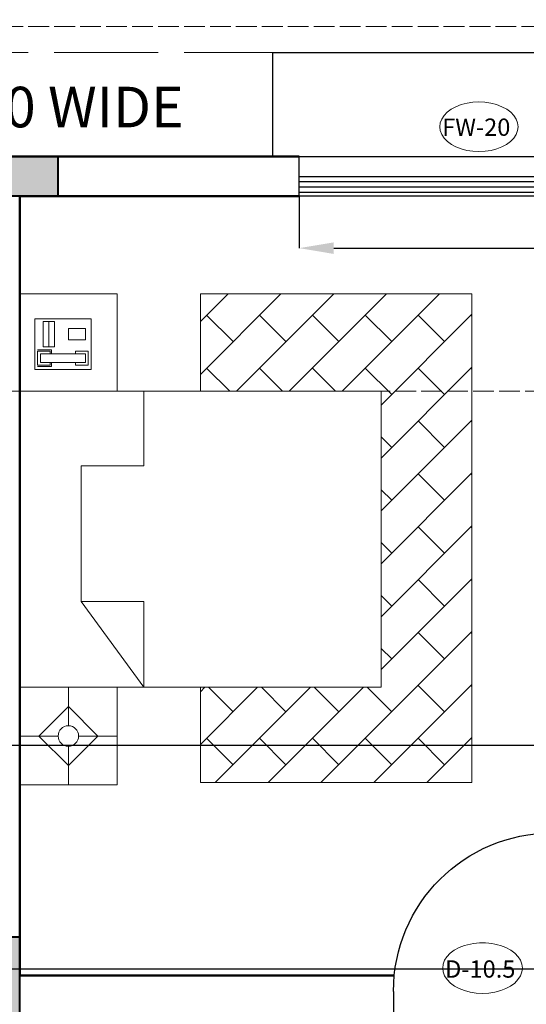
# Model space of a CAD drawing. Units: inches. Extents: x 22626 to 57351, y 2118 to 36234.
# Tile 8 of 10: x 41227 to 44155, y 23360 to 29046. Entities that reach past the tile are written whole.
import ezdxf

# ---------------------------------------------------------------- set-up
doc = ezdxf.new("R2010")
doc.units = ezdxf.units.IN
doc.header["$MEASUREMENT"] = 0
doc.linetypes.add('ACAD_ISO02W100', pattern=[15, 12, -3])
for name, color, linetype, lineweight in [('A-ANNO-DIMS', 130, 'Continuous', 18), ('A-ANNO-IDEN', 130, 'Continuous', 15), ('A-AREA-IDEN', 130, 'Continuous', 18), ('A-COLS', 7, 'Continuous', 40), ('A-ROOF', 80, 'Continuous', 25), ('A-ROOF-OVHD', 80, 'ACAD_ISO02W100', 18), ('A-WALL', 80, 'Continuous', 50), ('DOORS', 32, 'Continuous', 25), ('FURNITURE', 30, 'Continuous', 18), ('WINDOWS', 212, 'Continuous', 25)]:
    doc.layers.add(name, color=color, linetype=linetype, lineweight=lineweight)
doc.layers.add('A-SECT', color=2, linetype='ACAD_ISO02W100', lineweight=18, true_color=0xf1eb1f)
doc.styles.get("Standard").update_dxf_attribs({"font": 'arial.ttf'})
doc.dimstyles.get("Standard").update_dxf_attribs({"dimtxt": 150, "dimasz": 200, "dimexe": 0.18, "dimexo": 0.0625, "dimgap": 0.09, "dimtad": 0, "dimtih": 1, "dimtoh": 1, "dimdec": 0, "dimzin": 0, "dimdsep": 46, "dimtxsty": 'Standard', "dimcen": 0.09, "dimadec": 0, "dimazin": 0, "dimtfac": 1, "dimtdec": 0, "dimtofl": 0, "dimtmove": 0, "dimatfit": 3, "dimfxl": 1, "dimtolj": 1, "dimtzin": 0, "dimarcsym": 0})

# ---------------------------------------------------------------- blocks, each defined once
blk = doc.blocks.new('*U7')
for p, q in [((0, 0), (-1e-16, -5.999999999999999)), ((40, -6e-16), (40, -6))]:
    blk.add_line(p, q)
blk.add_lwpolyline([(0, 0), (5.6e-15, 40), (1.750000000000007, 40), (1.749999999999998, -7e-16)], close=True)
blk.add_arc((0, 0), 40, 0, 90)
blk = doc.blocks.new('Phone - Desk')
for p, q in [((-4.5, -5), (-4.5, 5)), ((-4.5, 5), (4.5, 5)), ((-4, 4.5), (-4, 2)), ((-3.75, 4.5), (-3.75, 2.25)), ((-1.25, 4.5), (-3.75, 4.5)), ((-3.25, 4), (-3.25, -4)), ((-3.25, 4), (-1.75, 4)), ((-1.75, -4), (-1.75, 4)), ((-1.25, 2.25), (-1.25, 4.5)), ((-1, 2), (-1, 4.5)), ((4, 3.5), (-0.5, 3.5)), ((-0.5, 3.5), (-0.5, 1.5)), ((4, 1.5), (4, 3.5)), ((4.5, 5), (4.5, -5)), ((-4, 2), (-3.25, 2)), ((-3.75, 2.25), (-3.25, 2.25)), ((-1.75, 2.25), (-1.25, 2.25)), ((-1.75, 2), (-1, 2)), ((-0.5, 2.5), (4, 2.5)), ((-0.5, 1.5), (4, 1.5)), ((2.75, -1), (0.75, -1)), ((0.75, -1), (0.75, -4)), ((2.75, -4), (2.75, -1)), ((-3.75, -2.25), (-3.25, -2.25)), ((-3.75, -4.5), (-3.75, -2.25)), ((-1.75, -2.25), (-1.25, -2.25)), ((-1.25, -2.25), (-1.25, -4.5)), ((4.5, -5), (-4.5, -5)), ((-1.25, -4.5), (-3.75, -4.5)), ((-3.25, -4), (-1.75, -4)), ((0.75, -4), (2.75, -4))]:
    blk.add_line(p, q)
blk = doc.blocks.new('BED')
h = blk.add_hatch()
h.set_pattern_fill('AR-B816', color=256, scale=27, angle=45)
h.set_pattern_definition([(45, (0, 0), (-152.7350647362943, 152.7350647362943), []), (135, (0, 0), (-305.4701294725885, 2.84e-14), [216, -216])])
h.paths.add_polyline_path([(36405.44497120028, 26900.74076162673), (36405.44497120028, 25190.72745343954), (35361.43700757947, 25190.72745343954), (35361.43700757947, 24640.23607026327), (36930.74850823512, 24640.23607026327), (36930.74850823512, 25190.72745343954), (36930.74850823512, 27463.39567013072), (36405.44497120028, 27463.39567013072), (35361.43700757947, 27463.39567013072), (35361.43700757947, 26900.74076162673)])
for p, q in [((35361.43700757947, 26900.74076162673), (35361.43700757947, 27463.39567013072)), ((35361.43700757947, 27463.39567013072), (36405.44497120028, 27463.39567013072)), ((36405.44497120028, 27463.39567013072), (36930.74850823512, 27463.39567013072)), ((36930.74850823512, 27463.39567013072), (36930.74850823512, 25190.72745343954)), ((35034.9123526114, 26900.74076162673), (35034.9123526114, 26469.4222770051)), ((34673.22155408209, 25686.2861194588), (34673.22155408209, 26469.4222770051)), ((35034.9123526114, 26469.4222770051), (34673.22155408209, 26469.4222770051)), ((35034.9123526114, 25686.2861194588), (34673.22155408209, 25686.2861194588)), ((34673.22155408209, 25686.2861194588), (35034.9123526114, 25190.72745343954)), ((35034.9123526114, 25190.72745343954), (35034.9123526114, 25686.2861194588)), ((34598.75649821064, 25190.72745343954), (34598.75649821064, 24968.41517241916)), ((35361.43700757947, 24640.23607026327), (35361.43700757947, 25190.72745343954)), ((36930.74850823512, 25190.72745343954), (36930.74850823512, 24640.23607026327)), ((34428.58518446884, 24909.39999918755), (34598.75649821064, 25079.57131292935)), ((34598.75649821064, 25079.57131292935), (34768.92781195245, 24909.39999918755)), ((34317.42904395865, 24909.39999918755), (34539.74132497903, 24909.39999918755)), ((34598.75649821065, 24739.22868544575), (34428.58518446884, 24909.39999918755)), ((34768.92781195245, 24909.39999918755), (34598.75649821065, 24739.22868544575)), ((34657.77167144226, 24909.39999918755), (34880.08395246263, 24909.39999918755)), ((34598.75649821065, 24850.38482595593), (34598.75649821064, 24628.07254493555)), ((36930.74850823512, 24640.23607026327), (35361.43700757947, 24640.23607026327))]:
    blk.add_line(p, q)
for points in [[(34317.42904395865, 26900.74076162673), (34880.08395246263, 26900.74076162673), (34880.08395246263, 27463.39567013072), (34317.42904395865, 27463.39567013072)], [(34317.42904395865, 26900.74076162673), (36405.44497120028, 26900.74076162673), (36405.44497120028, 25190.72745343954), (34317.42904395865, 25190.72745343954)], [(34317.42904395865, 25190.72745343954), (34880.08395246263, 25190.72745343954), (34880.08395246263, 24628.07254493555), (34317.42904395865, 24628.07254493555)]]:
    blk.add_lwpolyline(points, close=True)
blk.add_circle((34598.75649821064, 24909.39999918755), 59.01517323161534)
at = {"xscale": 32.52267765020765, "yscale": 32.52267765020765, "zscale": 32.52267765020765, "rotation": 90}
blk.add_blockref('Phone - Desk', (34566.99332919449, 27172.8579822775), dxfattribs=at)
blk = doc.blocks.new('WIN-FIXED-2000-REAR')
for p, q in [((4.39586510765e-05, 114.2630103577103), (2000.000043958651, 114.2630103577103)), ((4.39586510765e-05, 84.26301035771031), (2000.000043958651, 84.26301035771031)), ((4.39586510765e-05, 54.2630103577103), (2000.000043958651, 54.2630103577103)), ((4.39586510765e-05, 24.2630103577103), (2000.000043958651, 24.2630103577103))]:
    blk.add_line(p, q)
blk.add_lwpolyline([(4.39586510765e-05, 230.0001083647294), (2000.000043958651, 230.0001083647294), (2000.000043958651, 0.0001083647330233), (4.39586438006e-05, 0.0001083647330233), (4.39586510765e-05, 230.0001083647294)])
blk = doc.blocks.new('COL-RECTANGULAR')
h = blk.add_hatch(color=256)
h.dxf.hatch_style = 1
h.paths.add_polyline_path([(4.39586474386e-05, 0.0001083647293854), (450.0000439586474, 0.0001083647293854), (450.0000439586474, 230.0001083647294), (4.39586474386e-05, 230.0001083647294)])
blk.add_lwpolyline([(4.39586474386e-05, 0.0001083647293854), (4.39586474386e-05, 230.0001083647294), (450.0000439586474, 230.0001083647294), (450.0000439586474, 0.0001083647293854)], close=True)
blk = doc.blocks.new('WINDOW-HOOD')
for p, q in [((-0.0002120264252881, 0.0001083647293854), (-0.0002120264252881, 600.0001083647293)), ((-0.0002120264252881, 600.0001083647293), (2314.590014351226, 600.0001083647293)), ((2314.590014351226, 600.0001083647293), (2314.590014351226, 0.0001083647330233))]:
    blk.add_line(p, q)
blk = doc.blocks.new('*D82')
at = {"layer": 'A-ANNO-DIMS', "color": 0, "lineweight": -2, "transparency": 16777216}
for p, q in [((42842.42904395863, 28026.79760836474), (42842.42904395863, 27726.68010836474)), ((44842.42904395864, 28026.79760836474), (44842.42904395864, 27726.68010836474)), ((43042.42904395863, 27726.86010836474), (44642.42904395864, 27726.86010836474)), ((44842.42904395864, 27726.86010836474), (45042.42904395864, 27726.86010836474))]:
    blk.add_line(p, q, dxfattribs=at)
at = {"layer": 'A-ANNO-DIMS', "color": 0, "transparency": 16777216}
for points in [[(43042.42904395863, 27760.19344169807), (43042.42904395863, 27693.52677503141), (42842.42904395863, 27726.86010836474)], [(44642.42904395864, 27760.19344169807), (44642.42904395864, 27693.52677503141), (44842.42904395864, 27726.86010836474)]]:
    blk.add_solid(points, dxfattribs=at)
at = {"layer": 'Defpoints', "color": 0, "transparency": 16777216}
for p in [(42842.42904395863, 28026.86010836474), (44842.42904395864, 28026.86010836474), (44842.42904395864, 27726.86010836474)]:
    blk.add_point(p, dxfattribs=at)
at = {"layer": 'A-ANNO-DIMS', "color": 0, "transparency": 16777216, "insert": (46178.10908488633, 27726.86010836474), "char_height": 150, "attachment_point": 5}
blk.add_mtext('\\A1;REAR LIGHT 2000 TYP.', dxfattribs=at)
blk = doc.blocks.new('*D99')
at = {"layer": 'A-ANNO-DIMS', "color": 0, "lineweight": -2, "transparency": 16777216}
for p, q in [((41184.594559, 30456.86010800002), (57038.79342100006, 30456.86010800002)), ((57038.61342100005, 30256.86010800002), (57038.61342100005, 18933.58721577627)), ((57038.61342100006, 7456.860108000005), (57038.61342100005, 18780.13300022374)), ((43702.49154400001, 7256.860108000004), (57038.79342100006, 7256.860108000005))]:
    blk.add_line(p, q, dxfattribs=at)
at = {"layer": 'A-ANNO-DIMS', "color": 0, "transparency": 16777216}
for points in [[(57005.28008766672, 30256.86010800002), (57071.94675433339, 30256.86010800002), (57038.61342100005, 30456.86010800002)], [(57005.28008766673, 7456.860108000005), (57071.9467543334, 7456.860108000005), (57038.61342100006, 7256.860108000005)]]:
    blk.add_solid(points, dxfattribs=at)
at = {"layer": 'Defpoints', "color": 0, "transparency": 16777216}
for p in [(41184.53205900001, 30456.86010800002), (57038.61342100005, 30456.86010800002), (43702.42904400001, 7256.860108000004)]:
    blk.add_point(p, dxfattribs=at)
at = {"layer": 'A-ANNO-DIMS', "color": 0, "transparency": 16777216, "insert": (57038.61342100005, 18856.86010799999), "char_height": 150, "attachment_point": 5}
blk.add_mtext('\\A1;23200', dxfattribs=at)
blk = doc.blocks.new('*D109')
at = {"layer": 'A-ANNO-DIMS', "color": 0, "lineweight": -2, "transparency": 16777216}
for p, q in [((38641.09672300002, 24856.10781600001), (57038.79342100006, 24856.10781600002)), ((57038.61342100005, 24656.10781600002), (57038.61342100005, 24287.47888015827)), ((57038.61342100005, 23765.49804800001), (57038.61342100005, 24134.12698384176)), ((38641.09672300002, 23565.49804800001), (57038.79342100006, 23565.49804800001))]:
    blk.add_line(p, q, dxfattribs=at)
at = {"layer": 'A-ANNO-DIMS', "color": 0, "transparency": 16777216}
for points in [[(57005.28008766672, 24656.10781600002), (57071.94675433339, 24656.10781600002), (57038.61342100005, 24856.10781600002)], [(57005.28008766672, 23765.49804800001), (57071.94675433339, 23765.49804800001), (57038.61342100005, 23565.49804800001)]]:
    blk.add_solid(points, dxfattribs=at)
at = {"layer": 'Defpoints', "color": 0, "transparency": 16777216}
for p in [(38641.03422300002, 24856.10781600001), (57038.61342100005, 24856.10781600002), (38641.03422300002, 23565.49804800001)]:
    blk.add_point(p, dxfattribs=at)
at = {"layer": 'A-ANNO-DIMS', "color": 0, "transparency": 16777216, "insert": (57038.61342100005, 24210.802932), "char_height": 150, "attachment_point": 5}
blk.add_mtext('\\A1;1290.6', dxfattribs=at)

msp = doc.modelspace()

# ---------------------------------------------------------------- linework, layer by layer
at = {"layer": 'A-ANNO-IDEN'}
for centre, major_axis in [((43881.30460649732, 28427.77199422445), (226.1511443636677, 0)), ((43901.91556897389, 23568.93220751028), (230.2388321358037, 0))]:
    msp.add_ellipse(centre, major_axis=major_axis, ratio=0.6342549732601661, start_param=-1.570796326794896, end_param=4.712388980384689, dxfattribs=at)
at = {"layer": 'A-ROOF-OVHD', "ltscale": 10}
msp.add_lwpolyline([(33177.23707929009, 29006.86010836473), (33177.23707929009, 29006.86010836473), (48950.76462366981, 29006.86010836473), (48950.76462366981, 28256.86010836473)], dxfattribs=at)
at = {"layer": 'A-ROOF-OVHD', "ltscale": 50}
msp.add_lwpolyline([(33177.23707929009, 28256.86010836473), (33177.23707929009, 28856.86010836473), (48007.84353641211, 28856.86010836473), (48007.84353641211, 28256.86010836473)], dxfattribs=at)
at = {"layer": 'A-SECT', "ltscale": 10}
msp.add_line((55067.61444380648, 26900.74076162673), (24870.05537160907, 26900.74076162673), dxfattribs=at)
at = {"layer": 'A-WALL'}
for p, q in [((40097.42904395865, 28256.86010836473), (42842.42904395863, 28256.86010836473)), ((40997.42904395864, 28256.86010836473), (41447.42904395864, 28256.86010836473)), ((41227.42904395864, 28026.86010836473), (41227.42904395864, 23526.86010836473)), ((41227.42904395864, 28026.86010836473), (42842.42904395863, 28026.86010836474)), ((43392.14203564753, 23526.86010836473), (41227.42904395864, 23526.86010836473))]:
    msp.add_line(p, q, dxfattribs=at)

# ---------------------------------------------------------------- block references
at = {"layer": 'A-COLS'}
msp.add_blockref('COL-RECTANGULAR', (40997.42899999998, 28026.86), dxfattribs=at)
at = {"layer": 'A-COLS', "extrusion": (0, 0, -1), "zscale": -1, "rotation": 90}
msp.add_blockref('COL-RECTANGULAR', (-40997.4289355939, 23296.86006440608), dxfattribs=at)
at = {"layer": 'A-ROOF'}
msp.add_blockref('WINDOW-HOOD', (42689.76799999999, 28256.86), dxfattribs=at)
at = {"layer": 'DOORS', "xscale": -22.875, "yscale": 22.875, "zscale": 22.875}
msp.add_blockref('*U7', (44302.42904395864, 23434.11010836473), dxfattribs=at)
at = {"layer": 'FURNITURE'}
msp.add_blockref('BED', (6910, 0), dxfattribs=at)
at = {"layer": 'WINDOWS'}
msp.add_blockref('WIN-FIXED-2000-REAR', (42842.42899999999, 28026.86), dxfattribs=at)

# ---------------------------------------------------------------- texts
at = {"layer": 'A-ANNO-IDEN'}
for s, p in [('FW-20', (43668.86849377878, 28375.48962594912)), ('D-10.5', (43685.61761109566, 23513.6722529977))]:
    msp.add_text(s, height=100, dxfattribs=at).set_placement(p)
at = {"layer": 'A-AREA-IDEN'}
msp.add_text('OPEN PLAT FORM 1000 WIDE', height=234.52835186632, dxfattribs=at).set_placement((37895.41327221508, 28424.50343553665))

# ---------------------------------------------------------------- dimensions: what is measured, and where the dimension line sits
at = {"layer": 'A-ANNO-DIMS'}
for base, p1, p2, override, picture, middle in [((57038.61342100005, 30456.86010800002), (43702.42904399999, 7256.860107999999), (41184.53205899999, 30456.860108), {"dimdec": 0, "dimlfac": 1, "dimrnd": 0, "dimzin": 0, "dimdsep": 46, "dimlunit": 2}, '*D99', (57038.61342100005, 18856.86010799999)), ((57038.61342100005, 24856.10781600002), (38641.034223, 23565.498048), (38641.034223, 24856.107816), {"dimdec": 1, "dimlfac": 1, "dimrnd": 0, "dimzin": 0, "dimdsep": 46, "dimlunit": 2}, '*D109', (57038.61342100005, 24210.802932))]:
    dim = msp.add_linear_dim(base=base, p1=p1, p2=p2, angle=90, dimstyle='Standard', override=override, dxfattribs=at)
    dim.commit()
    dim.dimension.update_dxf_attribs({"geometry": picture, "text_midpoint": middle})
dim = msp.add_linear_dim(base=(44842.42904395864, 27726.86010836474), p1=(42842.42904395863, 28026.86010836474), p2=(44842.42904395864, 28026.86010836474), text='REAR LIGHT <> TYP.', dimstyle='Standard', override={"dimdec": 0, "dimlfac": 1, "dimrnd": 0, "dimzin": 0, "dimdsep": 46, "dimlunit": 2}, dxfattribs=at)
dim.commit()
dim.dimension.update_dxf_attribs({"geometry": '*D82', "text_midpoint": (46178.10908488633, 27726.86010836474)})

doc.saveas('drawing.dxf')
